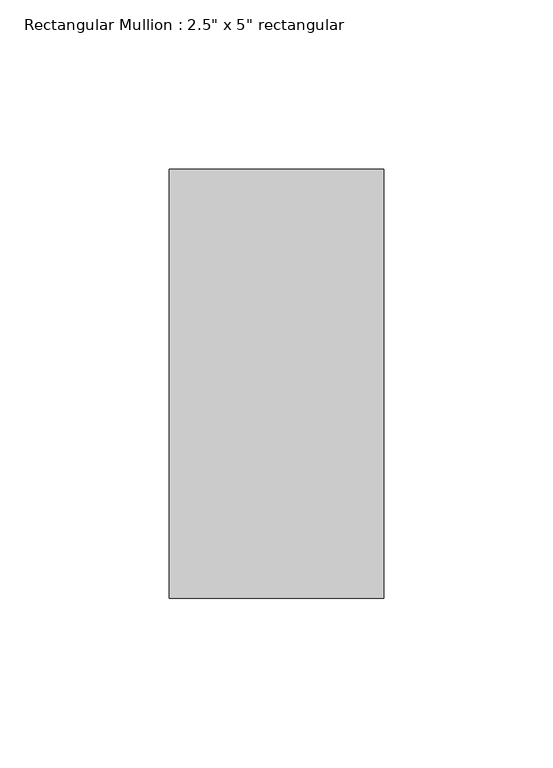
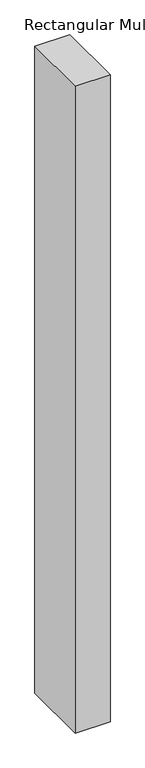
"""IFC4 building model written with IfcOpenShell, lengths in millimetres: member geometry."""

from ifc_helpers import new_model, si_unit, frame, origin, place, context, project, spatial, polyline, outline, extrude, source, transform, mapped, element, save


def member_71eb4692(model_context):
    return source(origin(), model_context, "Body", "SweptSolid", [
        extrude(outline(polyline([(0.0, 63.5), (0.0, -63.5), (-63.5, -63.5), (-63.5, 63.5), (0.0, 63.5)])), frame((0.0, 0.0, -1244.6), z_axis=(0.0, 0.0, 1.0), x_axis=(1.0, 0.0, 0.0)), (0.0, 0.0, 1.0), 1244.6),
    ])


if __name__ == "__main__":
    model = new_model("IFC4")
    model_context = context("Model", 3, world=origin())
    ifc_project = project(units=[si_unit("LENGTHUNIT", "METRE", prefix="MILLI")], contexts=[model_context])
    site = spatial("IfcSite", under=ifc_project)
    building = spatial("IfcBuilding", under=site)
    placement = place(None, origin())
    member_shape = member_71eb4692(model_context)
    element("IfcMember", 1, ObjectType="Rectangular Mullion : 2.5\" x 5\" rectangular", at=placement, inside=building, context=model_context, shape_type="MappedRepresentation", body=[
        mapped(member_shape, transform((0.0, 0.0, 0.0), x_axis=(1.0, 0.0, 0.0), y_axis=(0.0, 1.0, 0.0), z_axis=(0.0, 0.0, 1.0))),
    ])
    save(model, "model.ifc")

# Revit data of these elements
# Type "Rectangular Mullion : 2.5\" x 5\" rectangular"
#   built-in parameter 1007304 = 0.416667 (stored number, unit not read)
#   built-in parameter 1007301 = 0.104167 (stored number, unit not read)
#   built-in parameter 1007300 = 0.104167 (stored number, unit not read)
# Element 1 (IfcMember, "Rectangular Mullion : 2.5\" x 5\" rectangular")
#   Materials on its faces: "WINDOW FRAMING"
# Materials
#   "WINDOW FRAMING": class "Generic", colour RGB 120 120 120, transparency 0, Cost = 0
